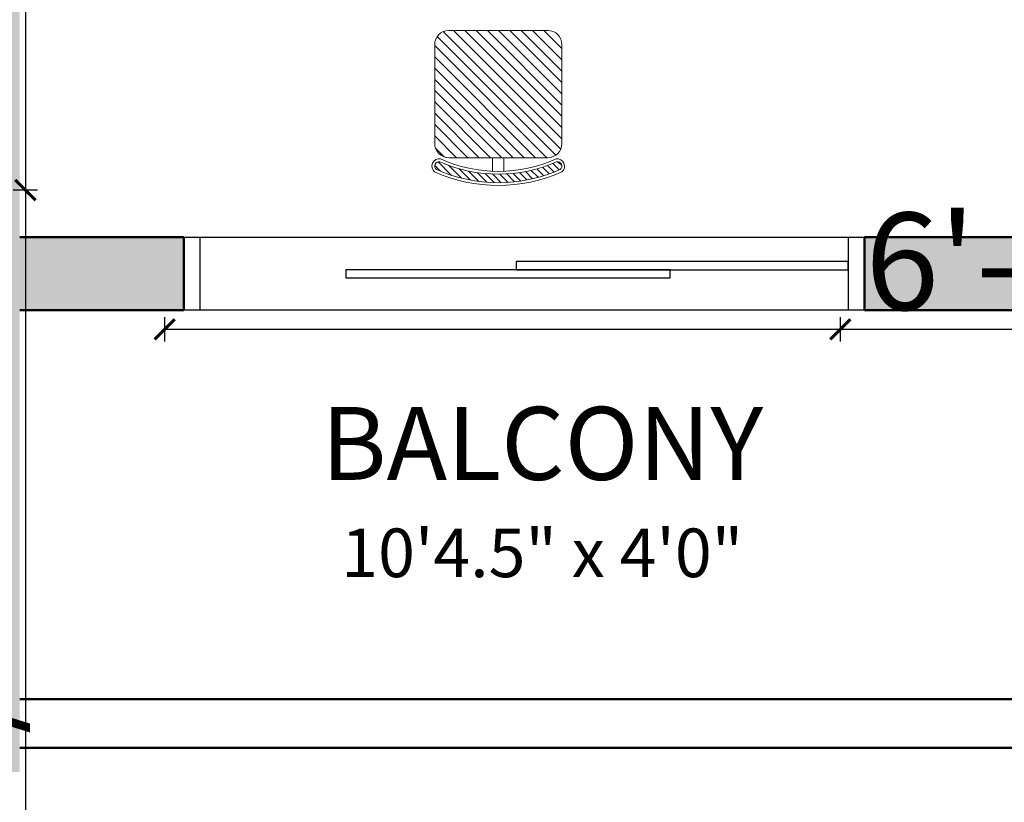
# Model space of a CAD drawing. Units: inches. Extents: x 375 to 1122, y 27 to 1069.
# Tile 7 of 155: x 667 to 788, y 157 to 253. Entities that reach past the tile are written whole.
import ezdxf

# ---------------------------------------------------------------- set-up
doc = ezdxf.new("R2010")
doc.units = ezdxf.units.IN
for name, color, linetype, lineweight in [('A-ANNO-DIMS', 2, 'Continuous', 18), ('A-AREA-IDEN', 7, 'Continuous', 18), ('A-COLS-PATT', 10, 'Continuous', 13), ('A-WALL-PATT', 252, 'Continuous', 13), ('Doors', 150, 'Continuous', 25), ('Furniture', 30, 'Continuous', 18), ('Walls', 250, 'Continuous', 50)]:
    doc.layers.add(name, color=color, linetype=linetype, lineweight=lineweight)
doc.styles.get("Standard").update_dxf_attribs({"font": 'arial.ttf'})
doc.dimstyles.new('ISO-25', dxfattribs={"dimtxt": 12, "dimasz": 2.5, "dimexe": 1.5, "dimexo": 1.5, "dimtad": 1, "dimdec": 1, "dimlunit": 3, "dimtxsty": 'Standard', "dimblk": 'ARCHTICK', "dimcen": 2.5, "dimadec": 0, "dimazin": 0, "dimtfac": 1, "dimtdec": 1, "dimtmove": 0, "dimatfit": 3, "dimfxl": 1.5, "dimfxlon": 1, "dimarcsym": 0})

# ---------------------------------------------------------------- blocks, each defined once
blk = doc.blocks.new('A$C403C54AD')
at = {"ltscale": 0.05}
for p, q in [((2.6911, 1.212, -0.0006), (2.3564, 0.8773, -0.0006)), ((2.6563, 1.212, -0.0006), (2.3564, 0.9121, -0.0006)), ((2.6215, 1.212, -0.0006), (2.3564, 0.9469, -0.0006)), ((2.5866, 1.212, -0.0006), (2.3564, 0.9818, -0.0006)), ((2.5518, 1.212, -0.0006), (2.3564, 1.0166, -0.0006)), ((2.517, 1.212, -0.0006), (2.3564, 1.0514, -0.0006)), ((2.4821, 1.212, -0.0006), (2.3564, 1.0862, -0.0006)), ((2.4473, 1.212, -0.0006), (2.3564, 1.1211, -0.0006)), ((2.4125, 1.212, -0.0006), (2.3564, 1.1559, -0.0006)), ((2.7225, 1.2085, -0.0006), (2.3599, 0.8459, -0.0006)), ((2.7416, 1.1928, -0.0006), (2.3756, 0.8268, -0.0006)), ((2.7734, 1.2115, -0.0006), (2.7615, 1.1996, -0.0006)), ((2.787, 1.2034, -0.0006), (2.767, 1.1834, -0.0006)), ((2.7934, 1.188, -0.0006), (2.7731, 1.1677, -0.0006)), ((2.7491, 1.1655, -0.0006), (2.4029, 0.8193, -0.0006)), ((2.7993, 1.1722, -0.0006), (2.7787, 1.1515, -0.0006)), ((2.8048, 1.1558, -0.0006), (2.7837, 1.1348, -0.0006)), ((2.7491, 1.1306, -0.0006), (2.4378, 0.8193, -0.0006)), ((2.8097, 1.139, -0.0006), (2.7882, 1.1175, -0.0006)), ((2.7491, 1.0958, -0.0006), (2.4726, 0.8193, -0.0006)), ((2.8141, 1.1216, -0.0006), (2.792, 1.0996, -0.0006)), ((2.8179, 1.1037, -0.0006), (2.7952, 1.081, -0.0006)), ((2.8211, 1.0851, -0.0006), (2.7977, 1.0617, -0.0006)), ((2.8236, 1.0658, -0.0006), (2.7993, 1.0415, -0.0006)), ((2.7491, 1.061, -0.0006), (2.5074, 0.8193, -0.0006)), ((2.8253, 1.0457, -0.0006), (2.8, 1.0205, -0.0006)), ((2.7491, 1.0262, -0.0006), (2.5422, 0.8193, -0.0006)), ((2.8261, 1.003, -0.0006), (2.7982, 0.9751, -0.0006)), ((2.8262, 1.0248, -0.0006), (2.7997, 0.9984, -0.0006)), ((2.7491, 0.9913, -0.0006), (2.5771, 0.8193, -0.0006)), ((2.8249, 0.98, -0.0006), (2.7952, 0.9504, -0.0006)), ((2.7491, 0.9565, -0.0006), (2.6119, 0.8193, -0.0006)), ((2.8224, 0.9558, -0.0006), (2.7904, 0.9238, -0.0006)), ((2.7491, 0.9217, -0.0006), (2.6467, 0.8193, -0.0006)), ((2.8184, 0.93, -0.0006), (2.7833, 0.8949, -0.0006)), ((2.7491, 0.8868, -0.0006), (2.6815, 0.8193, -0.0006)), ((2.8123, 0.9022, -0.0006), (2.7728, 0.8626, -0.0006)), ((2.8036, 0.8717, -0.0006), (2.7618, 0.8298, -0.0006)), ((2.7472, 0.8501, -0.0006), (2.7183, 0.8212, -0.0006)), ((2.791, 0.8373, -0.0006), (2.7733, 0.8196, -0.0006))]:
    blk.add_line(p, q, dxfattribs=at)
for p, q in [((2.7055, 1.212, -0.0006), (2.4001, 1.212, -0.0006)), ((2.3564, 1.1683, -0.0006), (2.3564, 0.8629, -0.0006)), ((2.7491, 0.8629, -0.0006), (2.7491, 1.1683, -0.0006)), ((2.7491, 1.0331, -0.0006), (2.7913, 1.0331, -0.0006)), ((2.7491, 0.9982, -0.0006), (2.7913, 0.9982, -0.0006)), ((2.4001, 0.8193, -0.0006), (2.531, 0.8193, -0.0006)), ((2.531, 0.8193, -0.0006), (2.7055, 0.8193, -0.0006))]:
    blk.add_line(p, q)
for centre, radius, start, end in [((2.7752, 1.1978, -0.0006), 0.0225, 38.8964, 189.6684), ((2.4001, 1.1683, -0.0006), 0.0436, 90, 180), ((2.7055, 1.1683, -0.0006), 0.0436, 0, 90), ((2.3575, 1.0156, -0.0006), 0.4338, 335.7176, 24.2824), ((2.3575, 1.0156, -0.0006), 0.4425, 335.7176, 24.2824), ((2.7752, 1.1978, -0.0006), 0.0138, 38.8964, 189.6684), ((2.3575, 1.0156, -0.0006), 0.4687, 335.7176, 24.2824), ((2.3575, 1.0156, -0.0006), 0.4774, 335.7176, 24.2824), ((2.4001, 0.8629, -0.0006), 0.0436, 180, 270), ((2.7055, 0.8629, -0.0006), 0.0436, 270, 0), ((2.7751, 0.8332, -0.0006), 0.0225, 169.7658, 321.6694), ((2.7751, 0.8332, -0.0006), 0.0138, 169.7658, 321.6694)]:
    blk.add_arc(centre, radius, start, end)
blk = doc.blocks.new('BALCONY-SLIDER-2P-84IN')
for points in [[(0, 9), (84, 9), (84, 0), (0, 0)], [(20, 4), (60, 4), (60, 5), (20, 5)], [(41, 5), (82, 5), (82, 6), (41, 6)]]:
    blk.add_lwpolyline(points, close=True)
for points in [[(2, 0), (2, 9)], [(82, 9), (82, 0)]]:
    blk.add_lwpolyline(points)
blk = doc.blocks.new('_ArchTick')
at = {"color": 0, "linetype": 'ByBlock', "const_width": 0.15}
blk.add_lwpolyline([(-0.5, -0.5), (0.5, 0.5)], dxfattribs=at)
blk = doc.blocks.new('*D59')
at = {"layer": 'A-ANNO-DIMS', "color": 0, "lineweight": -2, "transparency": 16777216}
for p, q in [((668.72, 346.85), (665.72, 346.85)), ((667.22, 346.85), (667.22, 232.35)), ((668.72, 232.35), (665.72, 232.35)), ((667.22, 232.35), (667.22, 27.5))]:
    blk.add_line(p, q, dxfattribs=at)
at = {"layer": 'Defpoints', "color": 0, "transparency": 16777216}
for p in [(684.39, 346.85), (667.22, 232.35), (684.39, 232.35)]:
    blk.add_point(p, dxfattribs=at)
at = {"layer": 'A-ANNO-DIMS', "color": 0, "lineweight": -2, "transparency": 16777216, "xscale": 2.5, "yscale": 2.5, "zscale": 2.5}
for p, rotation in [((667.22, 346.85), 90), ((667.22, 232.35), 270)]:
    blk.add_blockref('_ArchTick', p, dxfattribs=dict(at, rotation=rotation))
at = {"layer": 'A-ANNO-DIMS', "color": 0, "transparency": 16777216, "insert": (660.39, 128.67), "char_height": 12, "attachment_point": 5, "rotation": 90}
blk.add_mtext('DINING SET 9\'-6 1/2" TYP.', dxfattribs=at)
blk = doc.blocks.new('*D60')
at = {"layer": 'A-ANNO-DIMS', "color": 0, "lineweight": -2, "transparency": 16777216}
for p, q in [((684.39, 216.67), (684.39, 213.67)), ((767.77, 216.67), (767.77, 213.67)), ((684.39, 215.17), (767.77, 215.17)), ((767.77, 215.17), (882.02, 215.17))]:
    blk.add_line(p, q, dxfattribs=at)
at = {"layer": 'Defpoints', "color": 0, "transparency": 16777216}
for p in [(684.39, 232.35), (767.77, 232.35), (767.77, 215.17)]:
    blk.add_point(p, dxfattribs=at)
at = {"layer": 'A-ANNO-DIMS', "color": 0, "lineweight": -2, "transparency": 16777216, "xscale": 2.5, "yscale": 2.5, "zscale": 2.5, "rotation": 180}
blk.add_blockref('_ArchTick', (684.39, 215.17), dxfattribs=at)
at = {"layer": 'A-ANNO-DIMS', "color": 0, "lineweight": -2, "transparency": 16777216, "xscale": 2.5, "yscale": 2.5, "zscale": 2.5}
blk.add_blockref('_ArchTick', (767.77, 215.17), dxfattribs=at)
at = {"layer": 'A-ANNO-DIMS', "color": 0, "transparency": 16777216, "insert": (826.15, 222), "char_height": 12, "attachment_point": 5}
blk.add_mtext('6\'-11 1/2" TYP.', dxfattribs=at)
blk = doc.blocks.new('*D81')
at = {"layer": 'A-ANNO-DIMS', "color": 0, "lineweight": -2, "transparency": 16777216}
for p, q in [((444.51, 117.53), (444.51, 114.53)), ((989.01, 117.53), (989.01, 114.53)), ((444.51, 116.03), (989.01, 116.03))]:
    blk.add_line(p, q, dxfattribs=at)
at = {"layer": 'Defpoints', "color": 0, "transparency": 16777216}
for p in [(444.51, 187.53), (989.01, 187.53), (989.01, 116.03)]:
    blk.add_point(p, dxfattribs=at)
at = {"layer": 'A-ANNO-DIMS', "color": 0, "lineweight": -2, "transparency": 16777216, "xscale": 2.5, "yscale": 2.5, "zscale": 2.5, "rotation": 180}
blk.add_blockref('_ArchTick', (444.51, 116.03), dxfattribs=at)
at = {"layer": 'A-ANNO-DIMS', "color": 0, "lineweight": -2, "transparency": 16777216, "xscale": 2.5, "yscale": 2.5, "zscale": 2.5}
blk.add_blockref('_ArchTick', (989.01, 116.03), dxfattribs=at)
at = {"layer": 'A-ANNO-DIMS', "color": 0, "transparency": 16777216, "insert": (716.76, 122.86), "char_height": 12, "attachment_point": 5}
blk.add_mtext('45\'-4 1/2"', dxfattribs=at)
blk = doc.blocks.new('*D94')
at = {"layer": 'A-ANNO-DIMS', "color": 0, "lineweight": -2, "transparency": 16777216}
for p, q in [((734.01, 117.53), (734.01, 114.53)), ((773.01, 117.53), (773.01, 114.53)), ((734.01, 116.03), (773.01, 116.03))]:
    blk.add_line(p, q, dxfattribs=at)
at = {"layer": 'Defpoints', "color": 0, "transparency": 16777216}
for p in [(734.01, 667.53), (773.01, 667.53), (773.01, 116.03)]:
    blk.add_point(p, dxfattribs=at)
at = {"layer": 'A-ANNO-DIMS', "color": 0, "lineweight": -2, "transparency": 16777216, "xscale": 2.5, "yscale": 2.5, "zscale": 2.5, "rotation": 180}
blk.add_blockref('_ArchTick', (734.01, 116.03), dxfattribs=at)
at = {"layer": 'A-ANNO-DIMS', "color": 0, "lineweight": -2, "transparency": 16777216, "xscale": 2.5, "yscale": 2.5, "zscale": 2.5}
blk.add_blockref('_ArchTick', (773.01, 116.03), dxfattribs=at)
at = {"layer": 'A-ANNO-DIMS', "color": 0, "transparency": 16777216, "insert": (753.51, 122.78), "char_height": 12, "attachment_point": 5}
blk.add_mtext('3\'-3"', dxfattribs=at)

msp = doc.modelspace()

# ---------------------------------------------------------------- hatches: boundary and pattern name
at = {"layer": 'A-COLS-PATT'}
h = msp.add_hatch(color=256, dxfattribs=at)
h.dxf.hatch_style = 1
h.paths.add_polyline_path([(512.51, 982.53), (498.51, 982.53), (498.51, 973.53), (512.51, 973.53)])
h.paths.add_polyline_path([(666.51, 982.53), (652.51, 982.53), (652.51, 973.53), (666.51, 973.53)])
h.paths.add_polyline_path([(802.01, 982.53), (788.01, 982.53), (788.01, 973.53), (802.01, 973.53)])
h.paths.add_polyline_path([(932.01, 982.53), (918.01, 982.53), (918.01, 973.53), (932.01, 973.53)])
h.paths.add_polyline_path([(507.51, 841.53), (498.51, 841.53), (498.51, 827.53), (507.51, 827.53)])
h.paths.add_polyline_path([(666.51, 844.53), (652.51, 844.53), (652.51, 835.53), (666.51, 835.53)])
h.paths.add_polyline_path([(802.01, 814.53), (788.01, 814.53), (788.01, 805.53), (802.01, 805.53)])
h.paths.add_polyline_path([(932.01, 814.53), (918.01, 814.53), (918.01, 805.53), (932.01, 805.53)])
h.paths.add_polyline_path([(507.51, 719.53), (498.51, 719.53), (498.51, 705.53), (507.51, 705.53)])
h.paths.add_polyline_path([(731.01, 676.53), (722.01, 676.53), (722.01, 662.53), (731.01, 662.53)])
h.paths.add_polyline_path([(802.01, 676.53), (788.01, 676.53), (788.01, 667.53), (802.01, 667.53)])
h.paths.add_polyline_path([(932.01, 676.53), (918.01, 676.53), (918.01, 667.53), (932.01, 667.53)])
h.paths.add_polyline_path([(932.01, 583.53), (918.01, 583.53), (918.01, 574.53), (932.01, 574.53)])
h.paths.add_polyline_path([(868.01, 583.53), (854.01, 583.53), (854.01, 574.53), (868.01, 574.53)])
h.paths.add_polyline_path([(868.01, 502.53), (854.01, 502.53), (854.01, 493.53), (868.01, 493.53)])
h.paths.add_polyline_path([(932.01, 502.53), (918.01, 502.53), (918.01, 493.53), (932.01, 493.53)])
h.paths.add_polyline_path([(672.51, 592.03), (663.51, 592.03), (663.51, 578.03), (672.51, 578.03)])
h.paths.add_polyline_path([(512.51, 589.53), (498.51, 589.53), (498.51, 580.53), (512.51, 580.53)])
h.paths.add_polyline_path([(507.51, 464.53), (498.51, 464.53), (498.51, 450.53), (507.51, 450.53)])
h.paths.add_polyline_path([(731.01, 507.53), (722.01, 507.53), (722.01, 493.53), (731.01, 493.53)])
h.paths.add_polyline_path([(802.01, 502.53), (788.01, 502.53), (788.01, 493.53), (802.01, 493.53)])
h.paths.add_polyline_path([(507.51, 342.53), (498.51, 342.53), (498.51, 328.53), (507.51, 328.53)])
h.paths.add_polyline_path([(512.51, 196.53), (498.51, 196.53), (498.51, 187.53), (512.51, 187.53)])
h.paths.add_polyline_path([(666.51, 334.53), (652.51, 334.53), (652.51, 325.53), (666.51, 325.53)])
h.paths.add_polyline_path([(666.51, 196.53), (652.51, 196.53), (652.51, 187.53), (666.51, 187.53)])
h.paths.add_polyline_path([(805.01, 196.53), (791.01, 196.53), (791.01, 187.53), (805.01, 187.53)])
h.paths.add_polyline_path([(932.01, 196.53), (918.01, 196.53), (918.01, 187.53), (932.01, 187.53)])
h.paths.add_polyline_path([(932.01, 334.53), (918.01, 334.53), (918.01, 325.53), (932.01, 325.53)])
h.paths.add_polyline_path([(805.01, 334.53), (791.01, 334.53), (791.01, 325.53), (805.01, 325.53)])
at = {"layer": 'A-WALL-PATT'}
h = msp.add_hatch(color=256, dxfattribs=at)
h.dxf.hatch_style = 1
h.paths.add_polyline_path([(962.01, 388.53), (989.01, 388.53), (989.01, 394.53), (962.01, 394.53), (932.01, 394.53), (932.01, 397.53), (923.01, 397.53), (923.01, 394.53), (842.01, 394.53), (842.01, 334.53), (839.51, 334.53), (839.51, 328.53), (854.01, 328.53), (854.01, 334.53), (848.01, 334.53), (848.01, 388.53), (953.01, 388.53), (953.01, 356.08), (962.01, 356.08), (962.01, 358.55), (989.01, 358.55), (989.01, 364.55), (962.01, 364.55)])
h.paths.add_polyline_path([(989.01, 502.53), (932.01, 502.53), (932.01, 583.53), (932.01, 593.53), (923.01, 593.53), (923.01, 583.53), (854.01, 583.53), (854.01, 556.53), (863.01, 556.53), (863.01, 574.53), (923.01, 574.53), (923.01, 502.53), (863.01, 502.53), (863.01, 520.53), (854.01, 520.53), (854.01, 502.53), (773.01, 502.53), (773.01, 493.53), (788.01, 493.53), (788.01, 402.03), (722.01, 402.03), (722.01, 373.53), (728.01, 373.53), (728.01, 396.03), (788.01, 396.03), (788.01, 373.53), (794.01, 373.53), (794.01, 430.53), (814.01, 430.53), (814.01, 436.53), (794.01, 436.53), (794.01, 493.53), (923.01, 493.53), (923.01, 487.53), (932.01, 487.53), (932.01, 493.53), (983.01, 493.53), (983.01, 473.53), (989.01, 473.53)])
h.paths.add_polyline_path([(797.01, 325.53), (805.01, 325.53), (805.01, 328.53), (807.51, 328.53), (807.51, 334.53), (791.01, 334.53), (791.01, 226.53), (770.76, 226.53), (770.76, 217.53), (791.01, 217.53), (791.01, 187.53), (855.01, 187.53), (855.01, 196.53), (797.01, 196.53)])
h.paths.add_polyline_path([(989.01, 238.53), (962.01, 238.53), (962.01, 256.42), (953.01, 256.42), (953.01, 229.53), (980.01, 229.53), (980.01, 196.53), (915.01, 196.53), (915.01, 187.53), (989.01, 187.53)])
h.paths.add_polyline_path([(962.01, 334.53), (884.01, 334.53), (884.01, 328.53), (918.01, 328.53), (918.01, 325.53), (932.01, 325.53), (932.01, 328.53), (953.01, 328.53), (953.01, 304.42), (962.01, 304.42)])
h.paths.add_polyline_path([(606.51, 283.53), (609.51, 283.53), (609.51, 289.53), (600.51, 289.53), (600.51, 196.53), (578.51, 196.53), (578.51, 187.53), (606.51, 187.53), (606.51, 196.53)])
h.paths.add_polyline_path([(666.51, 292.53), (660.51, 292.53), (660.51, 289.53), (633.51, 289.53), (633.51, 283.53), (660.51, 283.53), (660.51, 196.53), (628.01, 196.53), (628.01, 187.53), (630.53, 187.53), (630.53, 160.53), (636.53, 160.53), (636.53, 187.53), (660.51, 187.53), (660.51, 160.53), (666.51, 160.53), (666.51, 217.53), (686.76, 217.53), (686.76, 226.53), (666.51, 226.53)])
h.paths.add_polyline_path([(480.51, 256.42), (471.51, 256.42), (471.51, 238.53), (444.51, 238.53), (444.51, 187.53), (518.51, 187.53), (518.51, 196.53), (453.51, 196.53), (453.51, 229.53), (480.51, 229.53)])
h.paths.add_polyline_path([(480.51, 328.53), (652.51, 328.53), (652.51, 325.53), (660.51, 325.53), (660.51, 322.53), (666.51, 322.53), (666.51, 334.53), (507.51, 334.53), (507.51, 360.53), (498.51, 360.53), (498.51, 334.53), (471.51, 334.53), (471.51, 304.42), (480.51, 304.42)])
h.paths.add_polyline_path([(507.51, 484.53), (498.51, 484.53), (498.51, 444.53), (507.51, 444.53), (507.51, 454.53), (621.51, 454.53), (621.51, 460.53), (507.51, 460.53)])
h.paths.add_polyline_path([(672.51, 604.53), (683.26, 604.53), (683.26, 613.53), (669.51, 613.53), (669.51, 649.53), (663.51, 649.53), (663.51, 589.53), (507.51, 589.53), (507.51, 613.53), (498.51, 613.53), (498.51, 556.53), (507.51, 556.53), (507.51, 580.53), (663.51, 580.53), (663.51, 520.53), (669.51, 520.53), (669.51, 556.53), (683.26, 556.53), (683.26, 565.53), (672.51, 565.53)])
h.paths.add_polyline_path([(731.01, 667.53), (734.01, 667.53), (734.01, 676.53), (728.01, 676.53), (728.01, 715.53), (657.51, 715.53), (657.51, 709.53), (663.51, 709.53), (663.51, 673.53), (669.51, 673.53), (669.51, 709.53), (722.01, 709.53), (722.01, 613.53), (704.76, 613.53), (704.76, 604.53), (722.01, 604.53), (722.01, 565.53), (704.76, 565.53), (704.76, 556.53), (722.01, 556.53), (722.01, 502.53), (722.01, 460.53), (669.51, 460.53), (669.51, 496.53), (663.51, 496.53), (663.51, 460.53), (657.51, 460.53), (657.51, 454.53), (728.01, 454.53), (728.01, 493.53), (734.01, 493.53), (734.01, 502.53), (731.01, 502.53)])
h.paths.add_polyline_path([(986.01, 718.53), (959.01, 718.53), (959.01, 727.53), (950.01, 727.53), (950.01, 709.53), (977.01, 709.53), (977.01, 676.53), (794.01, 676.53), (794.01, 805.53), (802.01, 805.53), (802.01, 808.53), (804.51, 808.53), (804.51, 814.53), (788.01, 814.53), (788.01, 774.03), (728.01, 774.03), (728.01, 796.53), (722.01, 796.53), (722.01, 768.03), (788.01, 768.03), (788.01, 676.53), (773.01, 676.53), (773.01, 667.53), (923.01, 667.53), (923.01, 657.53), (932.01, 657.53), (932.01, 667.53), (986.01, 667.53)])
h.paths.add_polyline_path([(621.51, 715.53), (507.51, 715.53), (507.51, 733.53), (498.51, 733.53), (498.51, 715.53), (498.51, 685.53), (507.51, 685.53), (507.51, 709.53), (621.51, 709.53)])
h.paths.add_polyline_path([(666.51, 847.03), (660.51, 847.03), (660.51, 844.53), (652.51, 844.53), (652.51, 841.53), (480.51, 841.53), (480.51, 859.53), (471.51, 859.53), (471.51, 835.53), (498.51, 835.53), (498.51, 817.53), (507.51, 817.53), (507.51, 835.53), (666.51, 835.53)])
h.paths.add_polyline_path([(480.51, 940.53), (453.51, 940.53), (453.51, 973.53), (518.51, 973.53), (518.51, 982.53), (444.51, 982.53), (444.51, 931.53), (471.51, 931.53), (471.51, 907.53), (480.51, 907.53)])
h.paths.add_polyline_path([(606.51, 982.53), (578.51, 982.53), (578.51, 973.53), (600.51, 973.53), (600.51, 880.53), (609.51, 880.53), (609.51, 886.53), (606.51, 886.53)])
h.paths.add_polyline_path([(666.51, 943.53), (686.76, 943.53), (686.76, 952.53), (666.51, 952.53), (666.51, 1009.53), (660.51, 1009.53), (660.51, 982.53), (636.53, 982.53), (636.53, 1009.53), (630.53, 1009.53), (630.53, 982.53), (628.01, 982.53), (628.01, 973.53), (660.51, 973.53), (660.51, 886.53), (633.51, 886.53), (633.51, 880.53), (660.51, 880.53), (660.51, 877.03), (666.51, 877.03)])
h.paths.add_polyline_path([(986.01, 874.53), (932.01, 874.53), (932.01, 877.53), (923.01, 877.53), (923.01, 874.53), (788.01, 874.53), (788.01, 868.53), (788.01, 844.53), (794.01, 844.53), (794.01, 868.53), (839.01, 868.53), (839.01, 814.53), (836.51, 814.53), (836.51, 808.53), (851.01, 808.53), (851.01, 814.53), (845.01, 814.53), (845.01, 868.53), (986.01, 868.53)])
h.paths.add_polyline_path([(959.01, 838.55), (986.01, 838.55), (986.01, 844.55), (959.01, 844.55), (959.01, 847.03), (950.01, 847.03), (950.01, 814.53), (881.01, 814.53), (881.01, 808.53), (918.01, 808.53), (918.01, 805.53), (932.01, 805.53), (932.01, 808.53), (950.01, 808.53), (950.01, 793.53), (959.01, 793.53)])
h.paths.add_polyline_path([(986.01, 982.53), (899.01, 982.53), (899.01, 973.53), (923.01, 973.53), (923.01, 967.53), (932.01, 967.53), (932.01, 973.53), (980.01, 973.53), (980.01, 953.53), (986.01, 953.53)])
h.paths.add_polyline_path([(851.01, 982.53), (788.01, 982.53), (788.01, 952.53), (770.76, 952.53), (770.76, 943.53), (788.01, 943.53), (788.01, 910.53), (814.01, 910.53), (814.01, 916.53), (794.01, 916.53), (794.01, 973.53), (851.01, 973.53)])

# ---------------------------------------------------------------- linework, layer by layer
at = {"layer": 'Walls'}
for p, q in [((686.76, 226.53), (666.51, 226.53)), ((686.76, 217.53), (686.76, 226.53)), ((791.01, 226.53), (770.76, 226.53)), ((770.76, 217.53), (770.76, 226.53)), ((686.76, 217.53), (666.51, 217.53)), ((791.01, 217.53), (770.76, 217.53)), ((791.01, 169.53), (666.51, 169.53)), ((797.01, 163.53), (666.51, 163.53))]:
    msp.add_line(p, q, dxfattribs=at)

# ---------------------------------------------------------------- block references
at = {"layer": 'Doors'}
msp.add_blockref('BALCONY-SLIDER-2P-84IN', (686.76, 217.53), dxfattribs=at)
at = {"layer": 'Furniture', "xscale": 39.9918517141215, "yscale": 39.9918517141215, "zscale": 39.9918517141215, "rotation": 270}
msp.add_blockref('A$C403C54AD', (684.95, 346.29, 0.02), dxfattribs=at)

# ---------------------------------------------------------------- texts
at = {"layer": 'A-AREA-IDEN', "insert": (697.93, 205.59), "char_height": 12, "attachment_point": 1}
msp.add_mtext_dynamic_manual_height_columns('\\pxqc;{\\fArial|b1|i0|c0|p34;\\H0.75x;BALCONY\\H1.33333x;\\P\\fArial|b0|i0|c0|p34;\\H0.5x;10\'4.5" x 4\'0"}', width=66.1169, gutter_width=12.5, heights=[0], dxfattribs=at)

# ---------------------------------------------------------------- dimensions: what is measured, and where the dimension line sits
at = {"layer": 'A-ANNO-DIMS'}
for base, p1, p2, picture, middle in [((773.01, 116.03), (734.01, 667.53), (773.01, 667.53), '*D94', (753.51, 122.78)), ((989.01, 116.03), (444.51, 187.53), (989.01, 187.53), '*D81', (716.76, 122.86))]:
    dim = msp.add_linear_dim(base=base, p1=p1, p2=p2, dimstyle='ISO-25', override={"dimdec": 1, "dimlfac": 1, "dimrnd": 0, "dimzin": 1, "dimdsep": 46, "dimlunit": 4, "dimfrac": 2}, dxfattribs=at)
    dim.commit()
    dim.dimension.update_dxf_attribs({"geometry": picture, "text_midpoint": middle})
dim = msp.add_linear_dim(base=(667.22, 232.35), p1=(684.39, 346.85), p2=(684.39, 232.35), angle=270, text='DINING SET <> TYP.', dimstyle='ISO-25', override={"dimdec": 1, "dimlfac": 1, "dimrnd": 0, "dimzin": 1, "dimdsep": 46, "dimlunit": 4, "dimfrac": 2}, dxfattribs=at)
dim.commit()
dim.dimension.update_dxf_attribs({"geometry": '*D59', "text_midpoint": (660.39, 128.67)})
dim = msp.add_linear_dim(base=(767.77, 215.17), p1=(684.39, 232.35), p2=(767.77, 232.35), text='<> TYP.', dimstyle='ISO-25', override={"dimdec": 1, "dimlfac": 1, "dimrnd": 0, "dimzin": 1, "dimdsep": 46, "dimlunit": 4, "dimfrac": 2}, dxfattribs=at)
dim.commit()
dim.dimension.update_dxf_attribs({"geometry": '*D60', "text_midpoint": (826.15, 222)})

doc.saveas('drawing.dxf')
